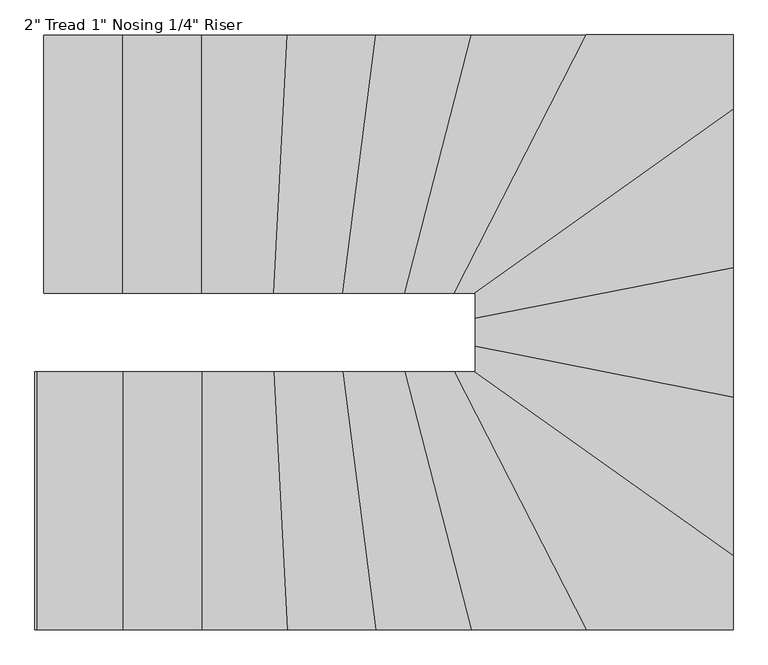
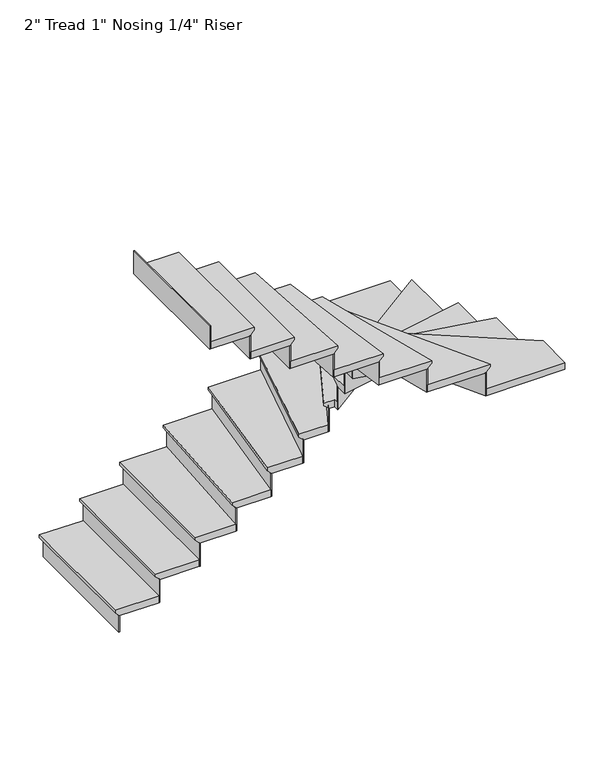
"""IFC4 building model written with IfcOpenShell, lengths in millimetres: stair flight geometry."""

from ifc_helpers import new_model, si_unit, origin, place, context, project, spatial, faceted_brep, source, transform, mapped, element, save


def stair_flight_927ef07f(model_context):
    return source(origin(), model_context, "Body", "Brep", [
        faceted_brep([(-3966.7570938, 382.5007235, 150.2833333), (-3966.7570938, 382.5007235, 169.3333333), (-3966.7570938, 1296.9007235, 169.3333333), (-3966.7570938, 1296.9007235, 150.2833333), (-3941.3570938, 382.5007235, 124.8833333), (-3941.3570938, 1296.9007235, 124.8833333), (-3661.9570938, 382.5007235, 169.3333333), (-3661.9570938, 1296.9007235, 169.3333333), (-3941.3570938, 1296.9007235, 118.5333333), (-3661.9570938, 1296.9007235, 118.5333333), (-3661.9570938, 382.5007235, 118.5333333), (-3941.3570938, 382.5007235, 118.5333333)], [[[0, 1, 2, 3]], [[4, 0, 3, 5]], [[2, 1, 6, 7]], [[8, 9, 10, 11]], [[2, 7, 9, 8, 5, 3]], [[8, 11, 4, 5]], [[6, 1, 0, 4, 11, 10]], [[7, 6, 10, 9]]]),
        faceted_brep([(-3941.3570938, 382.5007235, 118.5333333), (-3941.3570938, 382.5007235, 0.0), (-3935.0070938, 382.5007235, 0.0), (-3935.0070938, 382.5007235, 118.5333333), (-3941.3570938, 1296.9007235, 118.5333333), (-3935.0070938, 1296.9007235, 118.5333333), (-3935.0070938, 1296.9007235, 0.0), (-3941.3570938, 1296.9007235, 0.0)], [[[0, 1, 2, 3]], [[4, 5, 6, 7]], [[1, 0, 4, 7]], [[2, 1, 7, 6]], [[3, 2, 6, 5]], [[0, 3, 5, 4]]]),
        faceted_brep([(-3661.9570938, 382.5007235, 287.8666667), (-3661.9570938, 382.5007235, 118.5333333), (-3655.6070938, 382.5007235, 118.5333333), (-3655.6070938, 382.5007235, 287.8666667), (-3661.9570938, 1296.9007235, 287.8666667), (-3655.6070938, 1296.9007235, 287.8666667), (-3655.6070938, 1296.9007235, 118.5333333), (-3661.9570938, 1296.9007235, 118.5333333)], [[[0, 1, 2, 3]], [[4, 5, 6, 7]], [[1, 0, 4, 7]], [[2, 1, 7, 6]], [[3, 2, 6, 5]], [[0, 3, 5, 4]]]),
        faceted_brep([(-3687.3570938, 1296.9007235, 338.6666667), (-3687.3570938, 382.5007235, 338.6666667), (-3382.5570938, 382.5007235, 338.6666667), (-3382.5570938, 1296.9007235, 338.6666667), (-3661.9570938, 1296.9007235, 287.8666667), (-3382.5570938, 1296.9007235, 287.8666667), (-3382.5570938, 382.5007235, 287.8666667), (-3661.9570938, 382.5007235, 287.8666667), (-3661.9570938, 1296.9007235, 294.2166667), (-3687.3570938, 1296.9007235, 319.6166667), (-3661.9570938, 382.5007235, 294.2166667), (-3687.3570938, 382.5007235, 319.6166667)], [[[0, 1, 2, 3]], [[4, 5, 6, 7]], [[0, 3, 5, 4, 8, 9]], [[4, 7, 10, 8]], [[2, 1, 11, 10, 7, 6]], [[3, 2, 6, 5]], [[11, 1, 0, 9]], [[10, 11, 9, 8]]]),
        faceted_brep([(-3382.5570938, 382.5007235, 457.2), (-3382.5570938, 382.5007235, 287.8666667), (-3376.2070938, 382.5007235, 287.8666667), (-3376.2070938, 382.5007235, 457.2), (-3382.5570938, 1296.9007235, 457.2), (-3376.2070938, 1296.9007235, 457.2), (-3376.2070938, 1296.9007235, 287.8666667), (-3382.5570938, 1296.9007235, 287.8666667)], [[[0, 1, 2, 3]], [[4, 5, 6, 7]], [[1, 0, 4, 7]], [[2, 1, 7, 6]], [[3, 2, 6, 5]], [[0, 3, 5, 4]]]),
        faceted_brep([(-3407.9570938, 1296.9007235, 508.0), (-3407.9570938, 382.5007235, 508.0), (-3126.8899323, 382.5007235, 508.0), (-3079.3556619, 1296.9007235, 508.0), (-3382.5570938, 1296.9007235, 457.2), (-3079.3556619, 1296.9007235, 457.2), (-3126.8899323, 382.5007235, 457.2), (-3382.5570938, 382.5007235, 457.2), (-3382.5570938, 1296.9007235, 463.55), (-3407.9570938, 1296.9007235, 488.95), (-3382.5570938, 382.5007235, 463.55), (-3407.9570938, 382.5007235, 488.95)], [[[0, 1, 2, 3]], [[4, 5, 6, 7]], [[0, 3, 5, 4, 8, 9]], [[4, 7, 10, 8]], [[2, 1, 11, 10, 7, 6]], [[3, 2, 6, 5]], [[11, 1, 0, 9]], [[10, 11, 9, 8]]]),
        faceted_brep([(-3126.8899323, 382.5007235, 626.5333333), (-3126.8899323, 382.5007235, 457.2), (-3120.5313582, 382.5007235, 457.2), (-3120.5313582, 382.5007235, 626.5333333), (-3079.3556619, 1296.9007235, 626.5333333), (-3072.9970878, 1296.9007235, 626.5333333), (-3072.9970878, 1296.9007235, 457.2), (-3079.3556619, 1296.9007235, 457.2)], [[[0, 1, 2, 3]], [[4, 5, 6, 7]], [[1, 0, 4, 7]], [[2, 1, 7, 6]], [[3, 2, 6, 5]], [[0, 3, 5, 4]]]),
        faceted_brep([(-3104.7899586, 1296.9007235, 677.3333333), (-3152.324229, 382.5007235, 677.3333333), (-2882.7232325, 382.5007235, 677.3333333), (-2764.3671808, 1296.9007235, 677.3333333), (-3079.3556619, 1296.9007235, 626.5333333), (-2764.3671808, 1296.9007235, 626.5333333), (-2882.7232325, 382.5007235, 626.5333333), (-3126.8899323, 382.5007235, 626.5333333), (-3079.3556619, 1296.9007235, 632.8833333), (-3104.7899586, 1296.9007235, 658.2833333), (-3126.8899323, 382.5007235, 632.8833333), (-3152.324229, 382.5007235, 658.2833333)], [[[0, 1, 2, 3]], [[4, 5, 6, 7]], [[0, 3, 5, 4, 8, 9]], [[4, 7, 10, 8]], [[2, 1, 11, 10, 7, 6]], [[3, 2, 6, 5]], [[11, 1, 0, 9]], [[10, 11, 9, 8]]]),
        faceted_brep([(-2882.7232325, 382.5007235, 795.8666667), (-2882.7232325, 382.5007235, 626.5333333), (-2876.3202607, 382.5007235, 626.5333333), (-2876.3202607, 382.5007235, 795.8666667), (-2764.3671808, 1296.9007235, 795.8666667), (-2757.9642091, 1296.9007235, 795.8666667), (-2757.9642091, 1296.9007235, 626.5333333), (-2764.3671808, 1296.9007235, 626.5333333)], [[[0, 1, 2, 3]], [[4, 5, 6, 7]], [[1, 0, 4, 7]], [[2, 1, 7, 6]], [[3, 2, 6, 5]], [[0, 3, 5, 4]]]),
        faceted_brep([(-2789.979068, 1296.9007235, 846.6666667), (-2908.3351196, 382.5007235, 846.6666667), (-2661.09601, 382.5007235, 846.6666667), (-2425.9655626, 1296.9007235, 846.6666667), (-2764.3671808, 1296.9007235, 795.8666667), (-2425.9655626, 1296.9007235, 795.8666667), (-2661.09601, 382.5007235, 795.8666667), (-2882.7232325, 382.5007235, 795.8666667), (-2764.3671808, 1296.9007235, 802.2166667), (-2789.979068, 1296.9007235, 827.6166667), (-2882.7232325, 382.5007235, 802.2166667), (-2908.3351196, 382.5007235, 827.6166667)], [[[0, 1, 2, 3]], [[4, 5, 6, 7]], [[0, 3, 5, 4, 8, 9]], [[4, 7, 10, 8]], [[2, 1, 11, 10, 7, 6]], [[3, 2, 6, 5]], [[11, 1, 0, 9]], [[10, 11, 9, 8]]]),
        faceted_brep([(-2661.09601, 382.5007235, 965.2), (-2661.09601, 382.5007235, 795.8666667), (-2654.5394332, 382.5007235, 795.8666667), (-2654.5394332, 382.5007235, 965.2), (-2425.9655626, 1296.9007235, 965.2), (-2419.4089858, 1296.9007235, 965.2), (-2419.4089858, 1296.9007235, 795.8666667), (-2425.9655626, 1296.9007235, 795.8666667)], [[[0, 1, 2, 3]], [[4, 5, 6, 7]], [[1, 0, 4, 7]], [[2, 1, 7, 6]], [[3, 2, 6, 5]], [[0, 3, 5, 4]]]),
        faceted_brep([(-2452.1918701, 1296.9007235, 1016.0), (-2687.3223175, 382.5007235, 1016.0), (-2484.7493739, 382.5007235, 1016.0), (-2015.9247526, 1296.9007235, 1016.0), (-2425.9655626, 1296.9007235, 965.2), (-2015.9247526, 1296.9007235, 965.2), (-2484.7493739, 382.5007235, 965.2), (-2661.09601, 382.5007235, 965.2), (-2425.9655626, 1296.9007235, 971.55), (-2452.1918701, 1296.9007235, 996.95), (-2661.09601, 382.5007235, 971.55), (-2687.3223175, 382.5007235, 996.95)], [[[0, 1, 2, 3]], [[4, 5, 6, 7]], [[0, 3, 5, 4, 8, 9]], [[4, 7, 10, 8]], [[2, 1, 11, 10, 7, 6]], [[3, 2, 6, 5]], [[11, 1, 0, 9]], [[10, 11, 9, 8]]]),
        faceted_brep([(-2484.7493739, 382.5007235, 1134.5333333), (-2484.7493739, 382.5007235, 965.2), (-2477.6133908, 382.5007235, 965.2), (-2477.6133908, 382.5007235, 1134.5333333), (-2015.9247526, 1296.9007235, 1134.5333333), (-2008.7887695, 1296.9007235, 1134.5333333), (-2008.7887695, 1296.9007235, 965.2), (-2015.9247526, 1296.9007235, 965.2)], [[[0, 1, 2, 3]], [[4, 5, 6, 7]], [[1, 0, 4, 7]], [[2, 1, 7, 6]], [[3, 2, 6, 5]], [[0, 3, 5, 4]]]),
        faceted_brep([(-1524.6254019, 1003.2195898, 1185.3333333), (-1524.6254019, 1296.9007235, 1185.3333333), (-2044.4686852, 1296.9007235, 1185.3333333), (-2513.2933065, 382.5007235, 1185.3333333), (-2439.0254019, 382.5007235, 1185.3333333), (-2439.0254019, 352.9456407, 1185.3333333), (-1524.6254019, 1296.9007235, 1134.5333333), (-1524.6254019, 1003.2195898, 1134.5333333), (-2439.0254019, 352.9456407, 1134.5333333), (-2439.0254019, 382.5007235, 1134.5333333), (-2484.7493739, 382.5007235, 1134.5333333), (-2015.9247526, 1296.9007235, 1134.5333333), (-2015.9247526, 1296.9007235, 1140.8833333), (-2044.4686852, 1296.9007235, 1166.2833333), (-2484.7493739, 382.5007235, 1140.8833333), (-2513.2933065, 382.5007235, 1166.2833333)], [[[0, 1, 2, 3, 4, 5]], [[6, 7, 8, 9, 10, 11]], [[1, 0, 7, 6]], [[2, 1, 6, 11, 12, 13]], [[11, 10, 14, 12]], [[4, 3, 15, 14, 10, 9]], [[5, 4, 9, 8]], [[0, 5, 8, 7]], [[15, 3, 2, 13]], [[14, 15, 13, 12]]]),
        faceted_brep([(-2439.0254019, 352.9456407, 1303.8666667), (-2439.0254019, 352.9456407, 1134.5333333), (-2439.0254019, 345.1536659, 1134.5333333), (-2439.0254019, 345.1536659, 1303.8666667), (-1524.6254019, 1003.2195898, 1303.8666667), (-1524.6254019, 995.427615, 1303.8666667), (-1524.6254019, 995.427615, 1134.5333333), (-1524.6254019, 1003.2195898, 1134.5333333)], [[[0, 1, 2, 3]], [[4, 5, 6, 7]], [[1, 0, 4, 7]], [[2, 1, 7, 6]], [[3, 2, 6, 5]], [[0, 3, 5, 4]]]),
        faceted_brep([(-1524.6254019, 1034.387489, 1354.6666667), (-2439.0254019, 384.1135398, 1354.6666667), (-2439.0254019, 266.4915536, 1354.6666667), (-1524.6254019, 446.7324099, 1354.6666667), (-1524.6254019, 1003.2195898, 1303.8666667), (-1524.6254019, 446.7324099, 1303.8666667), (-2439.0254019, 266.4915536, 1303.8666667), (-2439.0254019, 352.9456407, 1303.8666667), (-1524.6254019, 1003.2195898, 1310.2166667), (-1524.6254019, 1034.387489, 1335.6166667), (-2439.0254019, 352.9456407, 1310.2166667), (-2439.0254019, 384.1135398, 1335.6166667)], [[[0, 1, 2, 3]], [[4, 5, 6, 7]], [[0, 3, 5, 4, 8, 9]], [[4, 7, 10, 8]], [[2, 1, 11, 10, 7, 6]], [[3, 2, 6, 5]], [[11, 1, 0, 9]], [[10, 11, 9, 8]]]),
        faceted_brep([(-2439.0254019, 266.4915536, 1473.2), (-2439.0254019, 266.4915536, 1303.8666667), (-2439.0254019, 260.0193682, 1303.8666667), (-2439.0254019, 260.0193682, 1473.2), (-1524.6254019, 446.7324099, 1473.2), (-1524.6254019, 440.2602245, 1473.2), (-1524.6254019, 440.2602245, 1303.8666667), (-1524.6254019, 446.7324099, 1303.8666667)], [[[0, 1, 2, 3]], [[4, 5, 6, 7]], [[1, 0, 4, 7]], [[2, 1, 7, 6]], [[3, 2, 6, 5]], [[0, 3, 5, 4]]]),
        faceted_brep([(-1524.6254019, 472.6211517, 1524.0), (-2439.0254019, 292.3802953, 1524.0), (-2439.0254019, 167.3324099, 1524.0), (-1524.6254019, -12.9084464, 1524.0), (-1524.6254019, 446.7324099, 1473.2), (-1524.6254019, -12.9084464, 1473.2), (-2439.0254019, 167.3324099, 1473.2), (-2439.0254019, 266.4915536, 1473.2), (-1524.6254019, 446.7324099, 1479.55), (-1524.6254019, 472.6211517, 1504.95), (-2439.0254019, 266.4915536, 1479.55), (-2439.0254019, 292.3802953, 1504.95)], [[[0, 1, 2, 3]], [[4, 5, 6, 7]], [[0, 3, 5, 4, 8, 9]], [[4, 7, 10, 8]], [[2, 1, 11, 10, 7, 6]], [[3, 2, 6, 5]], [[11, 1, 0, 9]], [[10, 11, 9, 8]]]),
        faceted_brep([(-2439.0254019, 167.3324099, 1642.5333333), (-2439.0254019, 167.3324099, 1473.2), (-2439.0254019, 160.8602245, 1473.2), (-2439.0254019, 160.8602245, 1642.5333333), (-1524.6254019, -12.9084464, 1642.5333333), (-1524.6254019, -19.3806318, 1642.5333333), (-1524.6254019, -19.3806318, 1473.2), (-1524.6254019, -12.9084464, 1473.2)], [[[0, 1, 2, 3]], [[4, 5, 6, 7]], [[1, 0, 4, 7]], [[2, 1, 7, 6]], [[3, 2, 6, 5]], [[0, 3, 5, 4]]]),
        faceted_brep([(-1524.6254019, 12.9802953, 1693.3333333), (-2439.0254019, 193.2211517, 1693.3333333), (-2439.0254019, 103.1007235, 1693.3333333), (-2485.1208764, 103.1007235, 1693.3333333), (-1524.6254019, -579.9539412, 1693.3333333), (-1524.6254019, -12.9084464, 1642.5333333), (-1524.6254019, -579.9539412, 1642.5333333), (-2485.1208764, 103.1007235, 1642.5333333), (-2439.0254019, 103.1007235, 1642.5333333), (-2439.0254019, 167.3324099, 1642.5333333), (-1524.6254019, -12.9084464, 1648.8833333), (-1524.6254019, 12.9802953, 1674.2833333), (-2439.0254019, 167.3324099, 1648.8833333), (-2439.0254019, 193.2211517, 1674.2833333)], [[[0, 1, 2, 3, 4]], [[5, 6, 7, 8, 9]], [[0, 4, 6, 5, 10, 11]], [[5, 9, 12, 10]], [[2, 1, 13, 12, 9, 8]], [[3, 2, 8, 7]], [[4, 3, 7, 6]], [[13, 1, 0, 11]], [[12, 13, 11, 10]]]),
        faceted_brep([(-2485.1208764, 103.1007235, 1811.8666667), (-2485.1208764, 103.1007235, 1642.5333333), (-2496.0777689, 103.1007235, 1642.5333333), (-2496.0777689, 103.1007235, 1811.8666667), (-1524.6254019, -579.9539412, 1811.8666667), (-1524.6254019, -587.7459159, 1811.8666667), (-1524.6254019, -587.7459159, 1642.5333333), (-1524.6254019, -579.9539412, 1642.5333333)], [[[0, 1, 2, 3]], [[4, 5, 6, 7]], [[1, 0, 4, 7]], [[2, 1, 7, 6]], [[3, 2, 6, 5]], [[0, 3, 5, 4]]]),
        faceted_brep([(-2073.0126177, -811.2992765, 1862.6666667), (-1524.6254019, -811.2992765, 1862.6666667), (-1524.6254019, -548.786042, 1862.6666667), (-2441.2933065, 103.1007235, 1862.6666667), (-2541.837239, 103.1007235, 1862.6666667), (-1524.6254019, -811.2992765, 1811.8666667), (-2073.0126177, -811.2992765, 1811.8666667), (-2541.837239, 103.1007235, 1811.8666667), (-2485.1208764, 103.1007235, 1811.8666667), (-1524.6254019, -579.9539412, 1811.8666667), (-1524.6254019, -579.9539412, 1818.2166667), (-1524.6254019, -548.786042, 1843.6166667), (-2485.1208764, 103.1007235, 1818.2166667), (-2441.2933065, 103.1007235, 1843.6166667)], [[[0, 1, 2, 3, 4]], [[5, 6, 7, 8, 9]], [[1, 0, 6, 5]], [[2, 1, 5, 9, 10, 11]], [[9, 8, 12, 10]], [[4, 3, 13, 12, 8, 7]], [[0, 4, 7, 6]], [[13, 3, 2, 11]], [[12, 13, 11, 10]]]),
        faceted_brep([(-2541.837239, 103.1007235, 1981.2), (-2541.837239, 103.1007235, 1811.8666667), (-2548.9732221, 103.1007235, 1811.8666667), (-2548.9732221, 103.1007235, 1981.2), (-2073.0126177, -811.2992765, 1981.2), (-2080.1486008, -811.2992765, 1981.2), (-2080.1486008, -811.2992765, 1811.8666667), (-2073.0126177, -811.2992765, 1811.8666667)], [[[0, 1, 2, 3]], [[4, 5, 6, 7]], [[1, 0, 4, 7]], [[2, 1, 7, 6]], [[3, 2, 6, 5]], [[0, 3, 5, 4]]]),
        faceted_brep([(-2044.4686852, -811.2992765, 2032.0), (-2513.2933065, 103.1007235, 2032.0), (-2713.548625, 103.1007235, 2032.0), (-2478.4181775, -811.2992765, 2032.0), (-2073.0126177, -811.2992765, 1981.2), (-2478.4181775, -811.2992765, 1981.2), (-2713.548625, 103.1007235, 1981.2), (-2541.837239, 103.1007235, 1981.2), (-2073.0126177, -811.2992765, 1987.55), (-2044.4686852, -811.2992765, 2012.95), (-2541.837239, 103.1007235, 1987.55), (-2513.2933065, 103.1007235, 2012.95)], [[[0, 1, 2, 3]], [[4, 5, 6, 7]], [[0, 3, 5, 4, 8, 9]], [[4, 7, 10, 8]], [[2, 1, 11, 10, 7, 6]], [[3, 2, 6, 5]], [[11, 1, 0, 9]], [[10, 11, 9, 8]]]),
        faceted_brep([(-2713.548625, 103.1007235, 2150.5333333), (-2713.548625, 103.1007235, 1981.2), (-2720.1052018, 103.1007235, 1981.2), (-2720.1052018, 103.1007235, 2150.5333333), (-2478.4181775, -811.2992765, 2150.5333333), (-2484.9747544, -811.2992765, 2150.5333333), (-2484.9747544, -811.2992765, 1981.2), (-2478.4181775, -811.2992765, 1981.2)], [[[0, 1, 2, 3]], [[4, 5, 6, 7]], [[1, 0, 4, 7]], [[2, 1, 7, 6]], [[3, 2, 6, 5]], [[0, 3, 5, 4]]]),
        faceted_brep([(-2452.1918701, -811.2992765, 2201.3333333), (-2687.3223175, 103.1007235, 2201.3333333), (-2933.9470067, 103.1007235, 2201.3333333), (-2815.5909551, -811.2992765, 2201.3333333), (-2478.4181775, -811.2992765, 2150.5333333), (-2815.5909551, -811.2992765, 2150.5333333), (-2933.9470067, 103.1007235, 2150.5333333), (-2713.548625, 103.1007235, 2150.5333333), (-2478.4181775, -811.2992765, 2156.8833333), (-2452.1918701, -811.2992765, 2182.2833333), (-2713.548625, 103.1007235, 2156.8833333), (-2687.3223175, 103.1007235, 2182.2833333)], [[[0, 1, 2, 3]], [[4, 5, 6, 7]], [[0, 3, 5, 4, 8, 9]], [[4, 7, 10, 8]], [[2, 1, 11, 10, 7, 6]], [[3, 2, 6, 5]], [[11, 1, 0, 9]], [[10, 11, 9, 8]]]),
        faceted_brep([(-2933.9470067, 103.1007235, 2319.8666667), (-2933.9470067, 103.1007235, 2150.5333333), (-2940.3499785, 103.1007235, 2150.5333333), (-2940.3499785, 103.1007235, 2319.8666667), (-2815.5909551, -811.2992765, 2319.8666667), (-2821.9939269, -811.2992765, 2319.8666667), (-2821.9939269, -811.2992765, 2150.5333333), (-2815.5909551, -811.2992765, 2150.5333333)], [[[0, 1, 2, 3]], [[4, 5, 6, 7]], [[1, 0, 4, 7]], [[2, 1, 7, 6]], [[3, 2, 6, 5]], [[0, 3, 5, 4]]]),
        faceted_brep([(-2789.979068, -811.2992765, 2370.6666667), (-2908.3351196, 103.1007235, 2370.6666667), (-3177.7585257, 103.1007235, 2370.6666667), (-3130.2242552, -811.2992765, 2370.6666667), (-2815.5909551, -811.2992765, 2319.8666667), (-3130.2242552, -811.2992765, 2319.8666667), (-3177.7585257, 103.1007235, 2319.8666667), (-2933.9470067, 103.1007235, 2319.8666667), (-2815.5909551, -811.2992765, 2326.2166667), (-2789.979068, -811.2992765, 2351.6166667), (-2933.9470067, 103.1007235, 2326.2166667), (-2908.3351196, 103.1007235, 2351.6166667)], [[[0, 1, 2, 3]], [[4, 5, 6, 7]], [[0, 3, 5, 4, 8, 9]], [[4, 7, 10, 8]], [[2, 1, 11, 10, 7, 6]], [[3, 2, 6, 5]], [[11, 1, 0, 9]], [[10, 11, 9, 8]]]),
        faceted_brep([(-3177.7585257, 103.1007235, 2489.2), (-3177.7585257, 103.1007235, 2319.8666667), (-3184.1170998, 103.1007235, 2319.8666667), (-3184.1170998, 103.1007235, 2489.2), (-3130.2242552, -811.2992765, 2489.2), (-3136.5828294, -811.2992765, 2489.2), (-3136.5828294, -811.2992765, 2319.8666667), (-3130.2242552, -811.2992765, 2319.8666667)], [[[0, 1, 2, 3]], [[4, 5, 6, 7]], [[1, 0, 4, 7]], [[2, 1, 7, 6]], [[3, 2, 6, 5]], [[0, 3, 5, 4]]]),
        faceted_brep([(-3104.7899586, -811.2992765, 2540.0), (-3152.324229, 103.1007235, 2540.0), (-3433.3570938, 103.1007235, 2540.0), (-3433.3570938, -811.2992765, 2540.0), (-3130.2242552, -811.2992765, 2489.2), (-3433.3570938, -811.2992765, 2489.2), (-3433.3570938, 103.1007235, 2489.2), (-3177.7585257, 103.1007235, 2489.2), (-3130.2242552, -811.2992765, 2495.55), (-3104.7899586, -811.2992765, 2520.95), (-3177.7585257, 103.1007235, 2495.55), (-3152.324229, 103.1007235, 2520.95)], [[[0, 1, 2, 3]], [[4, 5, 6, 7]], [[0, 3, 5, 4, 8, 9]], [[4, 7, 10, 8]], [[2, 1, 11, 10, 7, 6]], [[3, 2, 6, 5]], [[11, 1, 0, 9]], [[10, 11, 9, 8]]]),
        faceted_brep([(-3433.3570938, 103.1007235, 2658.5333333), (-3433.3570938, 103.1007235, 2489.2), (-3439.7070938, 103.1007235, 2489.2), (-3439.7070938, 103.1007235, 2658.5333333), (-3433.3570938, -811.2992765, 2658.5333333), (-3439.7070938, -811.2992765, 2658.5333333), (-3439.7070938, -811.2992765, 2489.2), (-3433.3570938, -811.2992765, 2489.2)], [[[0, 1, 2, 3]], [[4, 5, 6, 7]], [[1, 0, 4, 7]], [[2, 1, 7, 6]], [[3, 2, 6, 5]], [[0, 3, 5, 4]]]),
        faceted_brep([(-3407.9570938, -811.2992765, 2709.3333333), (-3407.9570938, 103.1007235, 2709.3333333), (-3712.7570938, 103.1007235, 2709.3333333), (-3712.7570938, -811.2992765, 2709.3333333), (-3433.3570938, -811.2992765, 2658.5333333), (-3712.7570938, -811.2992765, 2658.5333333), (-3712.7570938, 103.1007235, 2658.5333333), (-3433.3570938, 103.1007235, 2658.5333333), (-3433.3570938, -811.2992765, 2664.8833333), (-3407.9570938, -811.2992765, 2690.2833333), (-3433.3570938, 103.1007235, 2664.8833333), (-3407.9570938, 103.1007235, 2690.2833333)], [[[0, 1, 2, 3]], [[4, 5, 6, 7]], [[0, 3, 5, 4, 8, 9]], [[4, 7, 10, 8]], [[2, 1, 11, 10, 7, 6]], [[3, 2, 6, 5]], [[11, 1, 0, 9]], [[10, 11, 9, 8]]]),
        faceted_brep([(-3712.7570938, 103.1007235, 2827.8666667), (-3712.7570938, 103.1007235, 2658.5333333), (-3719.1070938, 103.1007235, 2658.5333333), (-3719.1070938, 103.1007235, 2827.8666667), (-3712.7570938, -811.2992765, 2827.8666667), (-3719.1070938, -811.2992765, 2827.8666667), (-3719.1070938, -811.2992765, 2658.5333333), (-3712.7570938, -811.2992765, 2658.5333333)], [[[0, 1, 2, 3]], [[4, 5, 6, 7]], [[1, 0, 4, 7]], [[2, 1, 7, 6]], [[3, 2, 6, 5]], [[0, 3, 5, 4]]]),
        faceted_brep([(-3992.1570938, 103.1007235, 2997.2), (-3992.1570938, 103.1007235, 2827.8666667), (-3998.5070938, 103.1007235, 2827.8666667), (-3998.5070938, 103.1007235, 2997.2), (-3992.1570938, -811.2992765, 2997.2), (-3998.5070938, -811.2992765, 2997.2), (-3998.5070938, -811.2992765, 2827.8666667), (-3992.1570938, -811.2992765, 2827.8666667)], [[[0, 1, 2, 3]], [[4, 5, 6, 7]], [[1, 0, 4, 7]], [[2, 1, 7, 6]], [[3, 2, 6, 5]], [[0, 3, 5, 4]]]),
        faceted_brep([(-3687.3570938, -811.2992765, 2878.6666667), (-3687.3570938, 103.1007235, 2878.6666667), (-3992.1570938, 103.1007235, 2878.6666667), (-3992.1570938, -811.2992765, 2878.6666667), (-3712.7570938, -811.2992765, 2827.8666667), (-3992.1570938, -811.2992765, 2827.8666667), (-3992.1570938, 103.1007235, 2827.8666667), (-3712.7570938, 103.1007235, 2827.8666667), (-3712.7570938, -811.2992765, 2834.2166667), (-3687.3570938, -811.2992765, 2859.6166667), (-3712.7570938, 103.1007235, 2834.2166667), (-3687.3570938, 103.1007235, 2859.6166667)], [[[0, 1, 2, 3]], [[4, 5, 6, 7]], [[0, 3, 5, 4, 8, 9]], [[4, 7, 10, 8]], [[2, 1, 11, 10, 7, 6]], [[3, 2, 6, 5]], [[11, 1, 0, 9]], [[10, 11, 9, 8]]]),
    ])


if __name__ == "__main__":
    model = new_model("IFC4")
    model_context = context("Model", 3, world=origin())
    ifc_project = project(units=[si_unit("LENGTHUNIT", "METRE", prefix="MILLI")], contexts=[model_context])
    site = spatial("IfcSite", under=ifc_project)
    building = spatial("IfcBuilding", under=site)
    placement = place(None, origin())
    stair_flight_shape = stair_flight_927ef07f(model_context)
    element("IfcStairFlight", 1, ObjectType="2\" Tread 1\" Nosing 1/4\" Riser", at=placement, inside=building, context=model_context, shape_type="MappedRepresentation", body=[
        mapped(stair_flight_shape, transform((0.0, 0.0, 0.0), x_axis=(1.0, 0.0, 0.0), y_axis=(0.0, 1.0, 0.0), z_axis=(0.0, 0.0, 1.0))),
    ])
    save(model, "model.ifc")
